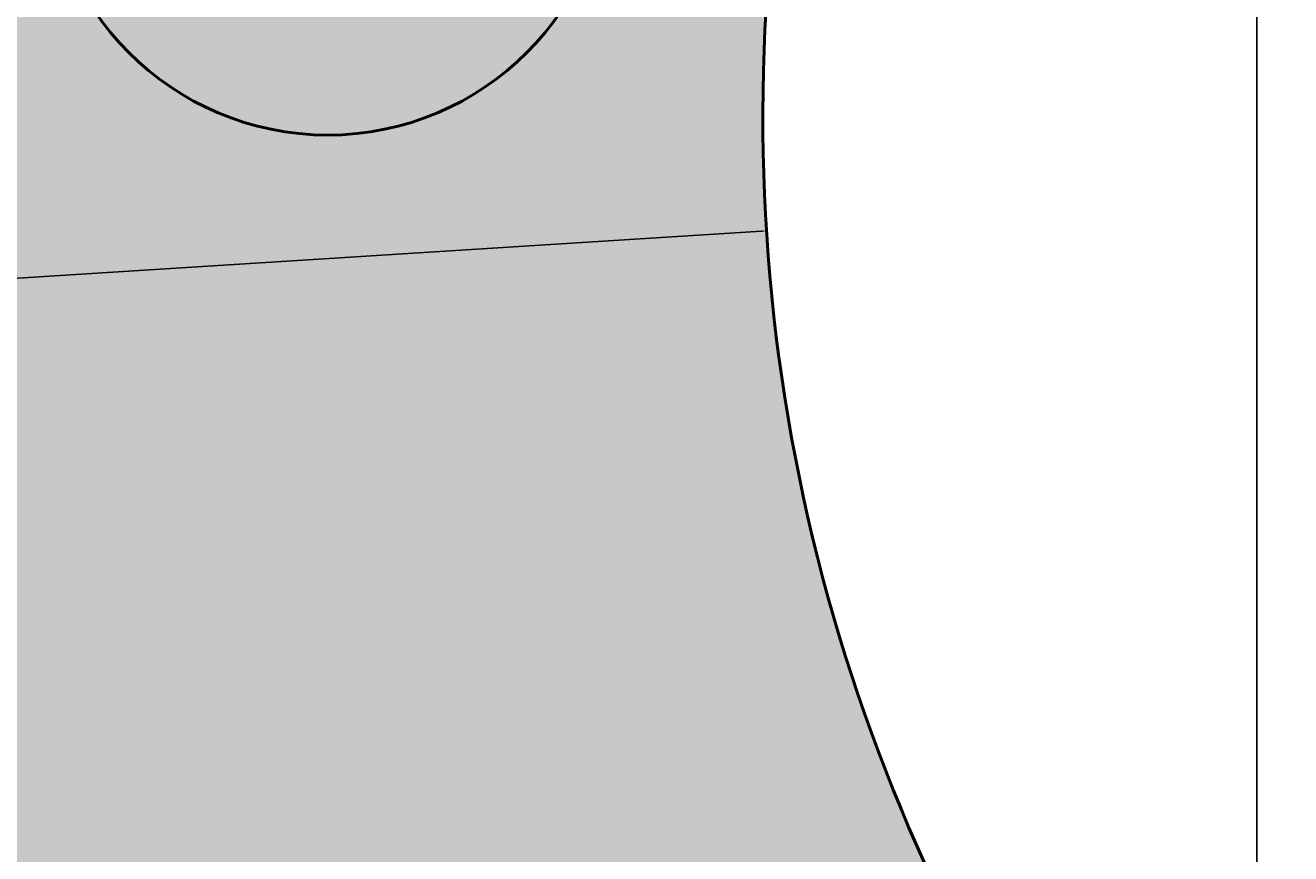
# Model space of a CAD drawing. Units: inches. Extents: x -13 to 107, y -48 to 102.
# Tile 11 of 13: x 17 to 62, y 43 to 72. Entities that reach past the tile are written whole.
import ezdxf

# ---------------------------------------------------------------- set-up
doc = ezdxf.new("R2010")
doc.units = ezdxf.units.IN
doc.header["$MEASUREMENT"] = 0
for name, color, linetype, lineweight in [('M-DIMS', 2, 'Continuous', 18), ('M-HATC', 8, 'Continuous', 18), ('M-OUTL', 7, 'Continuous', 50)]:
    doc.layers.add(name, color=color, linetype=linetype, lineweight=lineweight)
doc.styles.get("Standard").update_dxf_attribs({"font": 'arial.ttf'})
doc.dimstyles.get("Standard").update_dxf_attribs({"dimtxt": 0.18, "dimasz": 0.18, "dimexe": 0.18, "dimexo": 0.0625, "dimgap": 0.09, "dimtad": 0, "dimtih": 1, "dimtoh": 1, "dimdec": 4, "dimzin": 0, "dimdsep": 46, "dimtxsty": 'Standard', "dimcen": 0.09, "dimadec": 0, "dimazin": 0, "dimtfac": 1, "dimtdec": 4, "dimtofl": 0, "dimtmove": 0, "dimatfit": 3, "dimfxl": 1, "dimtolj": 1, "dimtzin": 0, "dimarcsym": 0})

# ---------------------------------------------------------------- blocks, each defined once
blk = doc.blocks.new('*D1')
at = {"layer": 'Defpoints', "color": 0, "transparency": 16777216}
for p in [(60.544, 101.543), (-5.45, 13.883), (60.544, 13.883)]:
    blk.add_point(p, dxfattribs=at)
at = {"layer": 'M-DIMS', "color": 0, "lineweight": -2, "transparency": 16777216}
for p, q in [((-5.45, 13.945), (-5.45, 101.723)), ((60.544, 13.945), (60.544, 101.723)), ((-5.27, 101.543), (27.328, 101.543)), ((60.364, 101.543), (27.766, 101.543))]:
    blk.add_line(p, q, dxfattribs=at)
at = {"layer": 'M-DIMS', "color": 0, "transparency": 16777216}
for points in [[(-5.27, 101.573), (-5.27, 101.513), (-5.45, 101.543)], [(60.364, 101.573), (60.364, 101.513), (60.544, 101.543)]]:
    blk.add_solid(points, dxfattribs=at)
at = {"layer": 'M-DIMS', "color": 0, "transparency": 16777216, "insert": (27.547, 101.543), "char_height": 0.18, "attachment_point": 5}
blk.add_mtext('\\A1;66', dxfattribs=at)
blk = doc.blocks.new('*D2')
at = {"layer": 'Defpoints', "color": 0, "transparency": 16777216}
for p in [(-12.585, 94.408), (27.547, 94.408), (27.547, -46.592)]:
    blk.add_point(p, dxfattribs=at)
at = {"layer": 'M-DIMS', "color": 0, "lineweight": -2, "transparency": 16777216}
for p, q in [((27.484, 94.408), (-12.765, 94.408)), ((-12.585, 94.228), (-12.585, 24.088)), ((-12.585, -46.412), (-12.585, 23.727)), ((27.484, -46.592), (-12.765, -46.592))]:
    blk.add_line(p, q, dxfattribs=at)
at = {"layer": 'M-DIMS', "color": 0, "transparency": 16777216}
for points in [[(-12.615, 94.228), (-12.555, 94.228), (-12.585, 94.408)], [(-12.615, -46.412), (-12.555, -46.412), (-12.585, -46.592)]]:
    blk.add_solid(points, dxfattribs=at)
at = {"layer": 'M-DIMS', "color": 0, "transparency": 16777216, "insert": (-12.585, 23.908), "char_height": 0.18, "attachment_point": 5}
blk.add_mtext('\\A1;141', dxfattribs=at)
blk = doc.blocks.new('*D4')
at = {"layer": 'Defpoints', "color": 0, "transparency": 16777216}
for p in [(27.547, 78.408), (67.679, 78.408), (27.547, 13.408)]:
    blk.add_point(p, dxfattribs=at)
at = {"layer": 'M-DIMS', "color": 0, "lineweight": -2, "transparency": 16777216}
for p, q in [((27.609, 78.408), (67.859, 78.408)), ((67.679, 78.228), (67.679, 46.09)), ((67.679, 13.588), (67.679, 45.726)), ((27.609, 13.408), (67.859, 13.408))]:
    blk.add_line(p, q, dxfattribs=at)
at = {"layer": 'M-DIMS', "color": 0, "transparency": 16777216}
for points in [[(67.649, 78.228), (67.709, 78.228), (67.679, 78.408)], [(67.649, 13.588), (67.709, 13.588), (67.679, 13.408)]]:
    blk.add_solid(points, dxfattribs=at)
at = {"layer": 'M-DIMS', "color": 0, "transparency": 16777216, "insert": (67.679, 45.908), "char_height": 0.18, "attachment_point": 5}
blk.add_mtext('\\A1;65', dxfattribs=at)
blk = doc.blocks.new('*D14')
at = {"layer": 'Defpoints', "color": 0, "transparency": 16777216}
for p in [(106.998, 69.054), (43.126, 65.005)]:
    blk.add_point(p, dxfattribs=at)
at = {"layer": 'M-DIMS', "color": 0, "lineweight": -2, "transparency": 16777216}
for p, q in [((106.908, 69.054), (107.088, 69.054)), ((106.998, 68.964), (106.998, 69.144)), ((4.803, 62.576), (42.947, 64.994))]:
    blk.add_line(p, q, dxfattribs=at)
at = {"layer": 'M-DIMS', "color": 0, "transparency": 16777216}
blk.add_solid([(42.945, 65.024), (42.949, 64.964), (43.126, 65.005)], dxfattribs=at)
at = {"layer": 'M-DIMS', "color": 0, "transparency": 16777216, "insert": (4.304, 62.576), "char_height": 0.18, "attachment_point": 5}
blk.add_mtext('\\A1;2X R64', dxfattribs=at)

msp = doc.modelspace()

# ---------------------------------------------------------------- hatches: boundary and pattern name
at = {"layer": 'M-HATC'}
h = msp.add_hatch(color=256, dxfattribs=at)
h.set_gradient(color1=(88, 186, 72), color2=(241, 235, 31), tint=1)
h.paths.add_polyline_path([(45.86, -14.044, 0.420873), (54.577, 32.339, -0.184081), (43.437, 76.537, 1.124637), (11.657, 76.537, -0.184081), (0.517, 32.339, 0.420873), (9.234, -14.044, -0.304084), (17.743, -34.622, 1.220926), (37.351, -34.622, -0.304084)])
h.paths.add_polyline_path([(33.479, -5.692, 0.859727), (21.615, -5.692, -0.111692), (13.972, -1.28, 0.859727), (8.04, 8.995, -0.111692), (8.04, 17.82, 0.859727), (13.972, 28.095, -0.111692), (21.615, 32.508, 0.859727), (33.479, 32.508, -0.111692), (41.122, 28.095, 0.859727), (47.054, 17.82, -0.111692), (47.054, 8.995, 0.859727), (41.122, -1.28, -0.111692)], flags=16)
h.paths.add_polyline_path([(32.547, -36.592, -1), (22.547, -36.592, -1)], flags=16)
h.paths.add_polyline_path([(17.547, 78.408, -1), (37.547, 78.408, -1)], flags=16)
h = msp.add_hatch(color=256, dxfattribs=at)
h.set_gradient(color1=(0, 0, 255), tint=1)
h.paths.add_polyline_path([(47.054, 8.995, 0.111692), (47.054, 17.82, -0.859727), (41.122, 28.095, 0.111692), (33.479, 32.508, -0.859727), (21.615, 32.508, 0.111692), (13.972, 28.095, -0.859727), (8.04, 17.82, 0.111692), (8.04, 8.995, -0.859727), (13.972, -1.28, 0.111692), (21.615, -5.692, -0.859727), (33.479, -5.692, 0.111692), (41.122, -1.28, -0.859727)])
h.paths.add_polyline_path([(37.547, 78.408, 1), (17.547, 78.408, 1)])
h.paths.add_polyline_path([(32.547, -36.592, 1), (22.547, -36.592, 1)])

# ---------------------------------------------------------------- linework, layer by layer
at = {"layer": 'M-OUTL'}
msp.add_circle((27.547, 78.408), 10, dxfattribs=at)
msp.add_arc((106.998, 69.054), 64, 173.28544, 215.00666, dxfattribs=at)

# ---------------------------------------------------------------- dimensions: what is measured, and where the dimension line sits
at = {"layer": 'M-DIMS'}
dim = msp.add_linear_dim(base=(60.544, 101.543), p1=(-5.45, 13.883), p2=(60.544, 13.883), dimstyle='Standard', override={"dimdec": 0, "dimlfac": 1, "dimrnd": 0, "dimzin": 0, "dimdsep": 46, "dimlunit": 2}, dxfattribs=at)
dim.commit()
dim.dimension.update_dxf_attribs({"geometry": '*D1', "text_midpoint": (27.547, 101.543)})
for base, p1, p2, picture, middle in [((-12.585, 94.408), (27.547, -46.592), (27.547, 94.408), '*D2', (-12.585, 23.908)), ((67.679, 78.408), (27.547, 13.408), (27.547, 78.408), '*D4', (67.679, 45.908))]:
    dim = msp.add_linear_dim(base=base, p1=p1, p2=p2, angle=90, dimstyle='Standard', override={"dimdec": 0, "dimlfac": 1, "dimrnd": 0, "dimzin": 0, "dimdsep": 46, "dimlunit": 2}, dxfattribs=at)
    dim.commit()
    dim.dimension.update_dxf_attribs({"geometry": picture, "text_midpoint": middle})
dim = msp.add_radius_dim(center=(106.998, 69.054), mpoint=(43.126, 65.005), text='2X <>', dimstyle='Standard', override={"dimdec": 0, "dimlfac": 1, "dimrnd": 0, "dimzin": 0, "dimdsep": 46, "dimlunit": 2}, dxfattribs=at)
dim.commit()
dim.dimension.update_dxf_attribs({"geometry": '*D14', "text_midpoint": (4.803, 62.576), "dimtype": 164})

doc.saveas('drawing.dxf')
